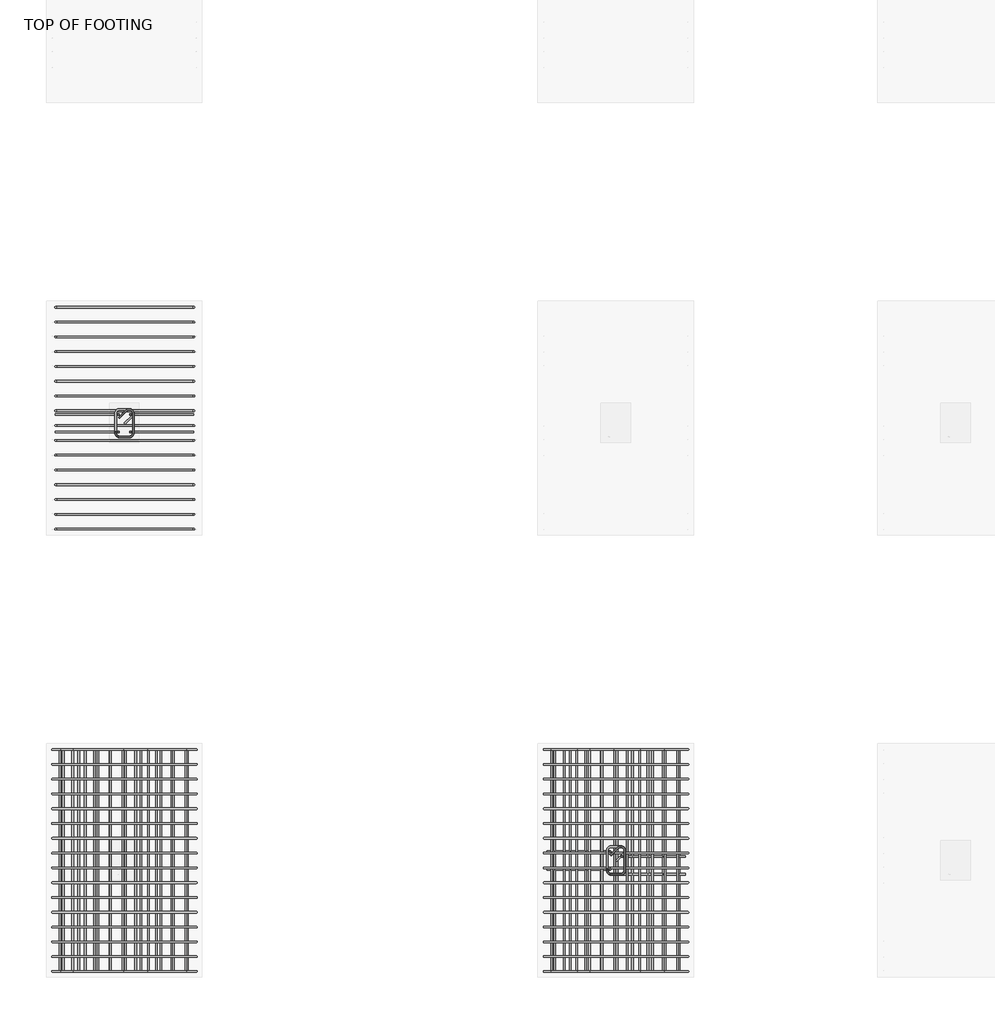
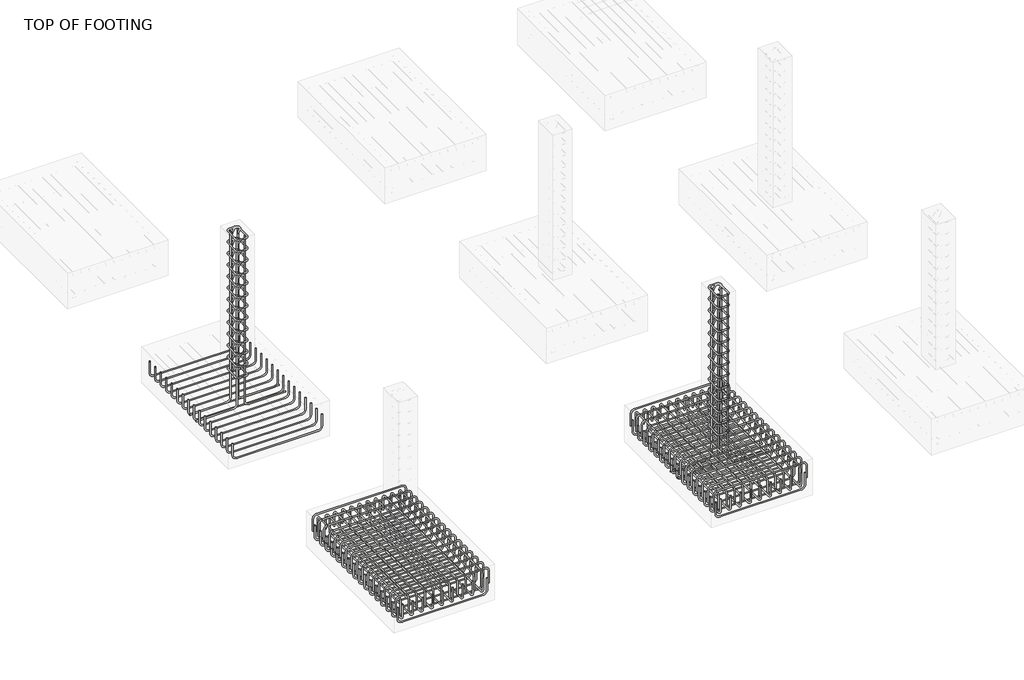
# One storey, part 5 of 8: 15 reinforcing bars.
"""IFC4 building model written with IfcOpenShell, lengths in millimetres."""

from ifc_helpers import new_model, si_unit, point, frame, origin, place, context, project, spatial, polyline, circle_curve, trimmed, segment, composite_curve, source, transform, mapped, element, save
from ifc_brep_helpers import swept_disk

model = new_model("IFC4")

# Units and contexts
model_context = context("Model", 3, world=origin())
ifc_project = project(units=[si_unit("LENGTHUNIT", "METRE", prefix="MILLI")], contexts=[model_context])

# Site, building, storey
site = spatial("IfcSite", under=ifc_project)
building = spatial("IfcBuilding", under=site)
storey = spatial("IfcBuildingStorey", under=building, Name="TOP OF FOOTING", Elevation=-1828.8)

# Reinforcing bars
placement = place(None, origin())
reinforcing_bar_shape = source(origin(), model_context, "Body", "SolidModel", [
    swept_disk(composite_curve([segment(polyline([(6846.0817577, 2235.4007933, -46.35), (6901.8253207, 2291.1443562, -46.35)]), True, "CONTINUOUS"), segment(trimmed(circle_curve(frame((6923.9931183, 2268.9765586, -46.35), z_axis=(0.0, 0.0, -1.0), x_axis=(-22.167797600000085, 22.167797600000085, 0.0)), 31.35), [point((6901.8253207, 2291.1443562, -46.35))], [point((6955.3431183, 2268.9765586, -46.35))], True, "CARTESIAN"), True, "CONTINUOUS"), segment(polyline([(6955.3431183, 2268.9765586, -46.35), (6955.3431183, 2119.5765586, -46.35)]), True, "CONTINUOUS"), segment(trimmed(circle_curve(frame((6923.9931183, 2119.5765586, -46.35), z_axis=(0.0, 0.0, -1.0), x_axis=(31.350000000000364, 0.0, 0.0)), 31.35), [point((6955.3431183, 2119.5765586, -46.35))], [point((6923.9931183, 2088.2265586, -46.35))], True, "CARTESIAN"), True, "CONTINUOUS"), segment(polyline([(6923.9931183, 2088.2265586, -46.35), (6850.7931183, 2088.2265586, -46.35)]), True, "CONTINUOUS"), segment(trimmed(circle_curve(frame((6850.7931183, 2119.5205096, -44.4761991), z_axis=(0.0, 0.05977036468717588, -0.9982121535551258), x_axis=(0.0, -31.293951000000106, -1.873800899999999)), 31.35), [point((6850.7931183, 2088.2265586, -46.35))], [point((6819.4431183, 2119.5205096, -44.4761991))], True, "CARTESIAN"), True, "CONTINUOUS"), segment(polyline([(6819.4431183, 2119.5205096, -44.4761991), (6819.4431183, 2269.0326076, -35.5238009)]), True, "CONTINUOUS"), segment(trimmed(circle_curve(frame((6850.7931183, 2269.0326076, -35.5238009), z_axis=(0.0, 0.05977036468717588, -0.9982121535551258), x_axis=(-31.350000000000364, 0.0, 0.0)), 31.35), [point((6819.4431183, 2269.0326076, -35.5238009))], [point((6850.7931183, 2300.3265586, -33.65))], True, "CARTESIAN"), True, "CONTINUOUS"), segment(polyline([(6850.7931183, 2300.3265586, -33.65), (6923.9931183, 2300.3265586, -33.65)]), True, "CONTINUOUS"), segment(trimmed(circle_curve(frame((6923.9931183, 2268.9765586, -33.65), z_axis=(0.0, 0.0, -1.0), x_axis=(0.0, 31.350000000000364, 0.0)), 31.35), [point((6923.9931183, 2300.3265586, -33.65))], [point((6946.1609159, 2246.808761, -33.65))], True, "CARTESIAN"), True, "CONTINUOUS"), segment(polyline([(6946.1609159, 2246.808761, -33.65), (6890.4173529, 2191.0651981, -33.65)]), True, "CONTINUOUS")], self_intersect=False), 6.35),
])
element("IfcReinforcingBar", 1, at=placement, inside=storey, context=model_context, shape_type="MappedRepresentation", body=[
    mapped(reinforcing_bar_shape, transform((0.0, 0.0, 0.0), x_axis=(1.0, 0.0, 0.0), y_axis=(0.0, 1.0, 0.0), z_axis=(0.0, 0.0, 1.0))),
    mapped(reinforcing_bar_shape, transform((0.0, 0.0, -144.675), x_axis=(1.0, 0.0, 0.0), y_axis=(0.0, 1.0, 0.0), z_axis=(0.0, 0.0, 1.0))),
    mapped(reinforcing_bar_shape, transform((0.0, 0.0, -289.35), x_axis=(1.0, 0.0, 0.0), y_axis=(0.0, 1.0, 0.0), z_axis=(0.0, 0.0, 1.0))),
    mapped(reinforcing_bar_shape, transform((0.0, 0.0, -434.025), x_axis=(1.0, 0.0, 0.0), y_axis=(0.0, 1.0, 0.0), z_axis=(0.0, 0.0, 1.0))),
    mapped(reinforcing_bar_shape, transform((0.0, 0.0, -578.7), x_axis=(1.0, 0.0, 0.0), y_axis=(0.0, 1.0, 0.0), z_axis=(0.0, 0.0, 1.0))),
    mapped(reinforcing_bar_shape, transform((0.0, 0.0, -723.375), x_axis=(1.0, 0.0, 0.0), y_axis=(0.0, 1.0, 0.0), z_axis=(0.0, 0.0, 1.0))),
    mapped(reinforcing_bar_shape, transform((0.0, 0.0, -868.05), x_axis=(1.0, 0.0, 0.0), y_axis=(0.0, 1.0, 0.0), z_axis=(0.0, 0.0, 1.0))),
    mapped(reinforcing_bar_shape, transform((0.0, 0.0, -1012.725), x_axis=(1.0, 0.0, 0.0), y_axis=(0.0, 1.0, 0.0), z_axis=(0.0, 0.0, 1.0))),
    mapped(reinforcing_bar_shape, transform((0.0, 0.0, -1157.4), x_axis=(1.0, 0.0, 0.0), y_axis=(0.0, 1.0, 0.0), z_axis=(0.0, 0.0, 1.0))),
    mapped(reinforcing_bar_shape, transform((0.0, 0.0, -1302.075), x_axis=(1.0, 0.0, 0.0), y_axis=(0.0, 1.0, 0.0), z_axis=(0.0, 0.0, 1.0))),
    mapped(reinforcing_bar_shape, transform((0.0, 0.0, -1446.75), x_axis=(1.0, 0.0, 0.0), y_axis=(0.0, 1.0, 0.0), z_axis=(0.0, 0.0, 1.0))),
    mapped(reinforcing_bar_shape, transform((0.0, 0.0, -1591.425), x_axis=(1.0, 0.0, 0.0), y_axis=(0.0, 1.0, 0.0), z_axis=(0.0, 0.0, 1.0))),
    mapped(reinforcing_bar_shape, transform((0.0, 0.0, -1736.1), x_axis=(1.0, 0.0, 0.0), y_axis=(0.0, 1.0, 0.0), z_axis=(0.0, 0.0, 1.0))),
])
reinforcing_bar_2_shape = source(origin(), model_context, "Body", "SolidModel", [
    swept_disk(composite_curve([segment(polyline([(7420.419602, 2088.2265586, -2177.1384798), (6979.2627797, 2088.2265586, -2177.1384798)]), True, "CONTINUOUS"), segment(trimmed(circle_curve(frame((6979.2627797, 2088.2265586, -2130.7884798), z_axis=(0.0, 1.0, 0.0), x_axis=(0.0, 0.0, -46.34999999999991)), 46.35), [point((6979.2627797, 2088.2265586, -2177.1384798))], [point((6932.9127797, 2088.2265586, -2130.7884798))], True, "CARTESIAN"), True, "CONTINUOUS"), segment(polyline([(6932.9127797, 2088.2265586, -2130.7884798), (6932.9127797, 2088.2265586, -40.0)]), True, "CONTINUOUS")], self_intersect=False), 6.35),
])
element("IfcReinforcingBar", 2, at=placement, inside=storey, context=model_context, shape_type="MappedRepresentation", body=[
    mapped(reinforcing_bar_2_shape, transform((0.0, 0.0, 0.0), x_axis=(1.0, 0.0, 0.0), y_axis=(0.0, 1.0, 0.0), z_axis=(0.0, 0.0, 1.0))),
    mapped(reinforcing_bar_2_shape, transform((0.0, 135.9, 0.0), x_axis=(1.0, 0.0, 0.0), y_axis=(0.0, 1.0, 0.0), z_axis=(0.0, 0.0, 1.0))),
])
reinforcing_bar_3_shape = source(origin(), model_context, "Body", "SolidModel", [
    swept_disk(composite_curve([segment(polyline([(6354.3666346, 2126.3265586, -2177.1384798), (6795.5234568, 2126.3265586, -2177.1384798)]), True, "CONTINUOUS"), segment(trimmed(circle_curve(frame((6795.5234568, 2126.3265586, -2130.7884798), z_axis=(0.0, -1.0, 0.0), x_axis=(0.0, 0.0, -46.34999999999991)), 46.35), [point((6795.5234568, 2126.3265586, -2177.1384798))], [point((6841.8734568, 2126.3265586, -2130.7884798))], True, "CARTESIAN"), True, "CONTINUOUS"), segment(polyline([(6841.8734568, 2126.3265586, -2130.7884798), (6841.8734568, 2126.3265586, -40.0)]), True, "CONTINUOUS")], self_intersect=False), 6.35),
])
element("IfcReinforcingBar", 3, at=placement, inside=storey, context=model_context, shape_type="MappedRepresentation", body=[
    mapped(reinforcing_bar_3_shape, transform((0.0, 0.0, 0.0), x_axis=(1.0, 0.0, 0.0), y_axis=(0.0, 1.0, 0.0), z_axis=(0.0, 0.0, 1.0))),
    mapped(reinforcing_bar_3_shape, transform((0.0, 135.9, 0.0), x_axis=(1.0, 0.0, 0.0), y_axis=(0.0, 1.0, 0.0), z_axis=(0.0, 0.0, 1.0))),
])
reinforcing_bar_4_shape = source(origin(), model_context, "Body", "SolidModel", [
    swept_disk(composite_curve([segment(polyline([(3061.4817577, 5600.7423139, -46.35), (3117.2253207, 5656.4858768, -46.35)]), True, "CONTINUOUS"), segment(trimmed(circle_curve(frame((3139.3931183, 5634.3180792, -46.35), z_axis=(0.0, 0.0, -1.0), x_axis=(-22.167797600000085, 22.167797600000085, 0.0)), 31.35), [point((3117.2253207, 5656.4858768, -46.35))], [point((3170.7431183, 5634.3180792, -46.35))], True, "CARTESIAN"), True, "CONTINUOUS"), segment(polyline([(3170.7431183, 5634.3180792, -46.35), (3170.7431183, 5484.9180792, -46.35)]), True, "CONTINUOUS"), segment(trimmed(circle_curve(frame((3139.3931183, 5484.9180792, -46.35), z_axis=(0.0, 0.0, -1.0), x_axis=(31.34999999999991, 0.0, 0.0)), 31.35), [point((3170.7431183, 5484.9180792, -46.35))], [point((3139.3931183, 5453.5680792, -46.35))], True, "CARTESIAN"), True, "CONTINUOUS"), segment(polyline([(3139.3931183, 5453.5680792, -46.35), (3066.1931183, 5453.5680792, -46.35)]), True, "CONTINUOUS"), segment(trimmed(circle_curve(frame((3066.1931183, 5484.8620303, -44.4761991), z_axis=(0.0, 0.05977036468717588, -0.9982121535551258), x_axis=(0.0, -31.293951099999504, -1.873800899999999)), 31.35), [point((3066.1931183, 5453.5680792, -46.35))], [point((3034.8431183, 5484.8620303, -44.4761991))], True, "CARTESIAN"), True, "CONTINUOUS"), segment(polyline([(3034.8431183, 5484.8620303, -44.4761991), (3034.8431183, 5634.3741282, -35.5238009)]), True, "CONTINUOUS"), segment(trimmed(circle_curve(frame((3066.1931183, 5634.3741282, -35.5238009), z_axis=(0.0, 0.05977036468717588, -0.9982121535551258), x_axis=(-31.350000000000364, 0.0, 0.0)), 31.35), [point((3034.8431183, 5634.3741282, -35.5238009))], [point((3066.1931183, 5665.6680792, -33.65))], True, "CARTESIAN"), True, "CONTINUOUS"), segment(polyline([(3066.1931183, 5665.6680792, -33.65), (3139.3931183, 5665.6680792, -33.65)]), True, "CONTINUOUS"), segment(trimmed(circle_curve(frame((3139.3931183, 5634.3180792, -33.65), z_axis=(0.0, 0.0, -1.0), x_axis=(0.0, 31.349999999999454, 0.0)), 31.35), [point((3139.3931183, 5665.6680792, -33.65))], [point((3161.5609159, 5612.1502816, -33.65))], True, "CARTESIAN"), True, "CONTINUOUS"), segment(polyline([(3161.5609159, 5612.1502816, -33.65), (3105.8173529, 5556.4067187, -33.65)]), True, "CONTINUOUS")], self_intersect=False), 6.35),
])
element("IfcReinforcingBar", 4, at=placement, inside=storey, context=model_context, shape_type="MappedRepresentation", body=[
    mapped(reinforcing_bar_4_shape, transform((0.0, 0.0, 0.0), x_axis=(1.0, 0.0, 0.0), y_axis=(0.0, 1.0, 0.0), z_axis=(0.0, 0.0, 1.0))),
    mapped(reinforcing_bar_4_shape, transform((0.0, 0.0, -144.675), x_axis=(1.0, 0.0, 0.0), y_axis=(0.0, 1.0, 0.0), z_axis=(0.0, 0.0, 1.0))),
    mapped(reinforcing_bar_4_shape, transform((0.0, 0.0, -289.35), x_axis=(1.0, 0.0, 0.0), y_axis=(0.0, 1.0, 0.0), z_axis=(0.0, 0.0, 1.0))),
    mapped(reinforcing_bar_4_shape, transform((0.0, 0.0, -434.025), x_axis=(1.0, 0.0, 0.0), y_axis=(0.0, 1.0, 0.0), z_axis=(0.0, 0.0, 1.0))),
    mapped(reinforcing_bar_4_shape, transform((0.0, 0.0, -578.7), x_axis=(1.0, 0.0, 0.0), y_axis=(0.0, 1.0, 0.0), z_axis=(0.0, 0.0, 1.0))),
    mapped(reinforcing_bar_4_shape, transform((0.0, 0.0, -723.375), x_axis=(1.0, 0.0, 0.0), y_axis=(0.0, 1.0, 0.0), z_axis=(0.0, 0.0, 1.0))),
    mapped(reinforcing_bar_4_shape, transform((0.0, 0.0, -868.05), x_axis=(1.0, 0.0, 0.0), y_axis=(0.0, 1.0, 0.0), z_axis=(0.0, 0.0, 1.0))),
    mapped(reinforcing_bar_4_shape, transform((0.0, 0.0, -1012.725), x_axis=(1.0, 0.0, 0.0), y_axis=(0.0, 1.0, 0.0), z_axis=(0.0, 0.0, 1.0))),
    mapped(reinforcing_bar_4_shape, transform((0.0, 0.0, -1157.4), x_axis=(1.0, 0.0, 0.0), y_axis=(0.0, 1.0, 0.0), z_axis=(0.0, 0.0, 1.0))),
    mapped(reinforcing_bar_4_shape, transform((0.0, 0.0, -1302.075), x_axis=(1.0, 0.0, 0.0), y_axis=(0.0, 1.0, 0.0), z_axis=(0.0, 0.0, 1.0))),
    mapped(reinforcing_bar_4_shape, transform((0.0, 0.0, -1446.75), x_axis=(1.0, 0.0, 0.0), y_axis=(0.0, 1.0, 0.0), z_axis=(0.0, 0.0, 1.0))),
    mapped(reinforcing_bar_4_shape, transform((0.0, 0.0, -1591.425), x_axis=(1.0, 0.0, 0.0), y_axis=(0.0, 1.0, 0.0), z_axis=(0.0, 0.0, 1.0))),
    mapped(reinforcing_bar_4_shape, transform((0.0, 0.0, -1736.1), x_axis=(1.0, 0.0, 0.0), y_axis=(0.0, 1.0, 0.0), z_axis=(0.0, 0.0, 1.0))),
])
reinforcing_bar_5_shape = source(origin(), model_context, "Body", "SolidModel", [
    swept_disk(composite_curve([segment(polyline([(3635.819602, 5491.6680792, -2177.1384798), (3194.6627797, 5491.6680792, -2177.1384798)]), True, "CONTINUOUS"), segment(trimmed(circle_curve(frame((3194.6627797, 5491.6680792, -2130.7884798), z_axis=(0.0, 1.0, 0.0), x_axis=(0.0, 0.0, -46.34999999999991)), 46.35), [point((3194.6627797, 5491.6680792, -2177.1384798))], [point((3148.3127797, 5491.6680792, -2130.7884798))], True, "CARTESIAN"), True, "CONTINUOUS"), segment(polyline([(3148.3127797, 5491.6680792, -2130.7884798), (3148.3127797, 5491.6680792, -40.0)]), True, "CONTINUOUS")], self_intersect=False), 6.35),
])
element("IfcReinforcingBar", 5, at=placement, inside=storey, context=model_context, shape_type="MappedRepresentation", body=[
    mapped(reinforcing_bar_5_shape, transform((0.0, 0.0, 0.0), x_axis=(1.0, 0.0, 0.0), y_axis=(0.0, 1.0, 0.0), z_axis=(0.0, 0.0, 1.0))),
    mapped(reinforcing_bar_5_shape, transform((0.0, 135.9, 0.0), x_axis=(1.0, 0.0, 0.0), y_axis=(0.0, 1.0, 0.0), z_axis=(0.0, 0.0, 1.0))),
])
reinforcing_bar_6_shape = source(origin(), model_context, "Body", "SolidModel", [
    swept_disk(composite_curve([segment(polyline([(2569.7666346, 5491.6680792, -2177.1384798), (3010.9234568, 5491.6680792, -2177.1384798)]), True, "CONTINUOUS"), segment(trimmed(circle_curve(frame((3010.9234568, 5491.6680792, -2130.7884798), z_axis=(0.0, -1.0, 0.0), x_axis=(0.0, 0.0, -46.34999999999991)), 46.35), [point((3010.9234568, 5491.6680792, -2177.1384798))], [point((3057.2734568, 5491.6680792, -2130.7884798))], True, "CARTESIAN"), True, "CONTINUOUS"), segment(polyline([(3057.2734568, 5491.6680792, -2130.7884798), (3057.2734568, 5491.6680792, -40.0)]), True, "CONTINUOUS")], self_intersect=False), 6.35),
])
element("IfcReinforcingBar", 6, at=placement, inside=storey, context=model_context, shape_type="MappedRepresentation", body=[
    mapped(reinforcing_bar_6_shape, transform((0.0, 0.0, 0.0), x_axis=(1.0, 0.0, 0.0), y_axis=(0.0, 1.0, 0.0), z_axis=(0.0, 0.0, 1.0))),
    mapped(reinforcing_bar_6_shape, transform((0.0, 135.9, 0.0), x_axis=(1.0, 0.0, 0.0), y_axis=(0.0, 1.0, 0.0), z_axis=(0.0, 0.0, 1.0))),
])
reinforcing_bar_7_shape = source(origin(), model_context, "Body", "SolidModel", [
    swept_disk(composite_curve([segment(polyline([(3637.0426771, 3047.9265586, -2008.2544267), (3637.0426771, 3047.9265586, -2155.5544267)]), True, "CONTINUOUS"), segment(trimmed(circle_curve(frame((3590.6926771, 3047.9265586, -2155.5544267), z_axis=(0.0, 1.0, 0.0), x_axis=(46.350000000000364, 0.0, 0.0)), 46.35), [point((3637.0426771, 3047.9265586, -2155.5544267))], [point((3590.6926771, 3047.9265586, -2201.9044267))], True, "CARTESIAN"), True, "CONTINUOUS"), segment(polyline([(3590.6926771, 3047.9265586, -2201.9044267), (2619.6766408, 3047.9265586, -2201.9044267)]), True, "CONTINUOUS"), segment(trimmed(circle_curve(frame((2619.6766408, 3047.9265586, -2155.5544267), z_axis=(0.0, 1.0, 0.0), x_axis=(0.0, 0.0, -46.34999999999991)), 46.35), [point((2619.6766408, 3047.9265586, -2201.9044267))], [point((2573.3266408, 3047.9265586, -2155.5544267))], True, "CARTESIAN"), True, "CONTINUOUS"), segment(polyline([(2573.3266408, 3047.9265586, -2155.5544267), (2573.3266408, 3047.9265586, -2008.2544267)]), True, "CONTINUOUS")], self_intersect=False), 6.35),
])
element("IfcReinforcingBar", 7, at=placement, inside=storey, context=model_context, shape_type="MappedRepresentation", body=[
    mapped(reinforcing_bar_7_shape, transform((0.0, 0.0, 0.0), x_axis=(1.0, 0.0, 0.0), y_axis=(0.0, 1.0, 0.0), z_axis=(0.0, 0.0, 1.0))),
    mapped(reinforcing_bar_7_shape, transform((0.0, -113.82, 0.0), x_axis=(1.0, 0.0, 0.0), y_axis=(0.0, 1.0, 0.0), z_axis=(0.0, 0.0, 1.0))),
    mapped(reinforcing_bar_7_shape, transform((0.0, -227.64, 0.0), x_axis=(1.0, 0.0, 0.0), y_axis=(0.0, 1.0, 0.0), z_axis=(0.0, 0.0, 1.0))),
    mapped(reinforcing_bar_7_shape, transform((0.0, -341.46, 0.0), x_axis=(1.0, 0.0, 0.0), y_axis=(0.0, 1.0, 0.0), z_axis=(0.0, 0.0, 1.0))),
    mapped(reinforcing_bar_7_shape, transform((0.0, -455.28, 0.0), x_axis=(1.0, 0.0, 0.0), y_axis=(0.0, 1.0, 0.0), z_axis=(0.0, 0.0, 1.0))),
    mapped(reinforcing_bar_7_shape, transform((0.0, -569.1, 0.0), x_axis=(1.0, 0.0, 0.0), y_axis=(0.0, 1.0, 0.0), z_axis=(0.0, 0.0, 1.0))),
    mapped(reinforcing_bar_7_shape, transform((0.0, -682.92, 0.0), x_axis=(1.0, 0.0, 0.0), y_axis=(0.0, 1.0, 0.0), z_axis=(0.0, 0.0, 1.0))),
    mapped(reinforcing_bar_7_shape, transform((0.0, -796.74, 0.0), x_axis=(1.0, 0.0, 0.0), y_axis=(0.0, 1.0, 0.0), z_axis=(0.0, 0.0, 1.0))),
    mapped(reinforcing_bar_7_shape, transform((0.0, -910.56, 0.0), x_axis=(1.0, 0.0, 0.0), y_axis=(0.0, 1.0, 0.0), z_axis=(0.0, 0.0, 1.0))),
    mapped(reinforcing_bar_7_shape, transform((0.0, -1024.38, 0.0), x_axis=(1.0, 0.0, 0.0), y_axis=(0.0, 1.0, 0.0), z_axis=(0.0, 0.0, 1.0))),
    mapped(reinforcing_bar_7_shape, transform((0.0, -1138.2, 0.0), x_axis=(1.0, 0.0, 0.0), y_axis=(0.0, 1.0, 0.0), z_axis=(0.0, 0.0, 1.0))),
    mapped(reinforcing_bar_7_shape, transform((0.0, -1252.02, 0.0), x_axis=(1.0, 0.0, 0.0), y_axis=(0.0, 1.0, 0.0), z_axis=(0.0, 0.0, 1.0))),
    mapped(reinforcing_bar_7_shape, transform((0.0, -1365.84, 0.0), x_axis=(1.0, 0.0, 0.0), y_axis=(0.0, 1.0, 0.0), z_axis=(0.0, 0.0, 1.0))),
    mapped(reinforcing_bar_7_shape, transform((0.0, -1479.66, 0.0), x_axis=(1.0, 0.0, 0.0), y_axis=(0.0, 1.0, 0.0), z_axis=(0.0, 0.0, 1.0))),
    mapped(reinforcing_bar_7_shape, transform((0.0, -1593.48, 0.0), x_axis=(1.0, 0.0, 0.0), y_axis=(0.0, 1.0, 0.0), z_axis=(0.0, 0.0, 1.0))),
    mapped(reinforcing_bar_7_shape, transform((0.0, -1707.3, 0.0), x_axis=(1.0, 0.0, 0.0), y_axis=(0.0, 1.0, 0.0), z_axis=(0.0, 0.0, 1.0))),
])
reinforcing_bar_8_shape = source(origin(), model_context, "Body", "SolidModel", [
    swept_disk(composite_curve([segment(polyline([(2549.1431183, 3047.9265586, -2068.8), (2549.1431183, 3047.9265586, -1921.5)]), True, "CONTINUOUS"), segment(trimmed(circle_curve(frame((2595.4931183, 3047.9265586, -1921.5), z_axis=(0.0, 1.0, 0.0), x_axis=(-46.34999999999991, 0.0, 0.0)), 46.35), [point((2549.1431183, 3047.9265586, -1921.5))], [point((2595.4931183, 3047.9265586, -1875.15))], True, "CARTESIAN"), True, "CONTINUOUS"), segment(polyline([(2595.4931183, 3047.9265586, -1875.15), (3610.0931183, 3047.9265586, -1875.15)]), True, "CONTINUOUS"), segment(trimmed(circle_curve(frame((3610.0931183, 3047.9265586, -1921.5), z_axis=(0.0, 1.0, 0.0), x_axis=(0.0, 0.0, 46.34999999999991)), 46.35), [point((3610.0931183, 3047.9265586, -1875.15))], [point((3656.4431183, 3047.9265586, -1921.5))], True, "CARTESIAN"), True, "CONTINUOUS"), segment(polyline([(3656.4431183, 3047.9265586, -1921.5), (3656.4431183, 3047.9265586, -2068.8)]), True, "CONTINUOUS")], self_intersect=False), 6.35),
])
element("IfcReinforcingBar", 8, at=placement, inside=storey, context=model_context, shape_type="MappedRepresentation", body=[
    mapped(reinforcing_bar_8_shape, transform((0.0, 0.0, 0.0), x_axis=(1.0, 0.0, 0.0), y_axis=(0.0, 1.0, 0.0), z_axis=(0.0, 0.0, 1.0))),
    mapped(reinforcing_bar_8_shape, transform((0.0, -113.82, 0.0), x_axis=(1.0, 0.0, 0.0), y_axis=(0.0, 1.0, 0.0), z_axis=(0.0, 0.0, 1.0))),
    mapped(reinforcing_bar_8_shape, transform((0.0, -227.64, 0.0), x_axis=(1.0, 0.0, 0.0), y_axis=(0.0, 1.0, 0.0), z_axis=(0.0, 0.0, 1.0))),
    mapped(reinforcing_bar_8_shape, transform((0.0, -341.46, 0.0), x_axis=(1.0, 0.0, 0.0), y_axis=(0.0, 1.0, 0.0), z_axis=(0.0, 0.0, 1.0))),
    mapped(reinforcing_bar_8_shape, transform((0.0, -455.28, 0.0), x_axis=(1.0, 0.0, 0.0), y_axis=(0.0, 1.0, 0.0), z_axis=(0.0, 0.0, 1.0))),
    mapped(reinforcing_bar_8_shape, transform((0.0, -569.1, 0.0), x_axis=(1.0, 0.0, 0.0), y_axis=(0.0, 1.0, 0.0), z_axis=(0.0, 0.0, 1.0))),
    mapped(reinforcing_bar_8_shape, transform((0.0, -682.92, 0.0), x_axis=(1.0, 0.0, 0.0), y_axis=(0.0, 1.0, 0.0), z_axis=(0.0, 0.0, 1.0))),
    mapped(reinforcing_bar_8_shape, transform((0.0, -796.74, 0.0), x_axis=(1.0, 0.0, 0.0), y_axis=(0.0, 1.0, 0.0), z_axis=(0.0, 0.0, 1.0))),
    mapped(reinforcing_bar_8_shape, transform((0.0, -910.56, 0.0), x_axis=(1.0, 0.0, 0.0), y_axis=(0.0, 1.0, 0.0), z_axis=(0.0, 0.0, 1.0))),
    mapped(reinforcing_bar_8_shape, transform((0.0, -1024.38, 0.0), x_axis=(1.0, 0.0, 0.0), y_axis=(0.0, 1.0, 0.0), z_axis=(0.0, 0.0, 1.0))),
    mapped(reinforcing_bar_8_shape, transform((0.0, -1138.2, 0.0), x_axis=(1.0, 0.0, 0.0), y_axis=(0.0, 1.0, 0.0), z_axis=(0.0, 0.0, 1.0))),
    mapped(reinforcing_bar_8_shape, transform((0.0, -1252.02, 0.0), x_axis=(1.0, 0.0, 0.0), y_axis=(0.0, 1.0, 0.0), z_axis=(0.0, 0.0, 1.0))),
    mapped(reinforcing_bar_8_shape, transform((0.0, -1365.84, 0.0), x_axis=(1.0, 0.0, 0.0), y_axis=(0.0, 1.0, 0.0), z_axis=(0.0, 0.0, 1.0))),
    mapped(reinforcing_bar_8_shape, transform((0.0, -1479.66, 0.0), x_axis=(1.0, 0.0, 0.0), y_axis=(0.0, 1.0, 0.0), z_axis=(0.0, 0.0, 1.0))),
    mapped(reinforcing_bar_8_shape, transform((0.0, -1593.48, 0.0), x_axis=(1.0, 0.0, 0.0), y_axis=(0.0, 1.0, 0.0), z_axis=(0.0, 0.0, 1.0))),
    mapped(reinforcing_bar_8_shape, transform((0.0, -1707.3, 0.0), x_axis=(1.0, 0.0, 0.0), y_axis=(0.0, 1.0, 0.0), z_axis=(0.0, 0.0, 1.0))),
])
reinforcing_bar_9_shape = source(origin(), model_context, "Body", "SolidModel", [
    swept_disk(composite_curve([segment(polyline([(2631.3651697, 3047.9265586, -1986.9111268), (2631.3651697, 3047.9265586, -2134.2111268)]), True, "CONTINUOUS"), segment(trimmed(circle_curve(frame((2631.3651697, 3001.5765586, -2134.2111268), z_axis=(-1.0, 0.0, 0.0), x_axis=(0.0, 46.34999999999991, 0.0)), 46.35), [point((2631.3651697, 3047.9265586, -2134.2111268))], [point((2631.3651697, 3001.5765586, -2180.5611268))], True, "CARTESIAN"), True, "CONTINUOUS"), segment(polyline([(2631.3651697, 3001.5765586, -2180.5611268), (2631.3651697, 1386.9765586, -2180.5611268)]), True, "CONTINUOUS"), segment(trimmed(circle_curve(frame((2631.3651697, 1386.9765586, -2134.2111268), z_axis=(-1.0, 0.0, 0.0), x_axis=(0.0, 0.0, -46.34999999999991)), 46.35), [point((2631.3651697, 1386.9765586, -2180.5611268))], [point((2631.3651697, 1340.6265586, -2134.2111268))], True, "CARTESIAN"), True, "CONTINUOUS"), segment(polyline([(2631.3651697, 1340.6265586, -2134.2111268), (2631.3651697, 1340.6265586, -1986.9111268)]), True, "CONTINUOUS")], self_intersect=False), 6.35),
])
element("IfcReinforcingBar", 9, at=placement, inside=storey, context=model_context, shape_type="MappedRepresentation", body=[
    mapped(reinforcing_bar_9_shape, transform((0.0, 0.0, 0.0), x_axis=(1.0, 0.0, 0.0), y_axis=(0.0, 1.0, 0.0), z_axis=(0.0, 0.0, 1.0))),
    mapped(reinforcing_bar_9_shape, transform((119.5564677, 0.0, 0.0), x_axis=(1.0, 0.0, 0.0), y_axis=(0.0, 1.0, 0.0), z_axis=(0.0, 0.0, 1.0))),
    mapped(reinforcing_bar_9_shape, transform((239.1129355, 0.0, 0.0), x_axis=(1.0, 0.0, 0.0), y_axis=(0.0, 1.0, 0.0), z_axis=(0.0, 0.0, 1.0))),
    mapped(reinforcing_bar_9_shape, transform((358.6694032, 0.0, 0.0), x_axis=(1.0, 0.0, 0.0), y_axis=(0.0, 1.0, 0.0), z_axis=(0.0, 0.0, 1.0))),
    mapped(reinforcing_bar_9_shape, transform((478.2258709, 0.0, 0.0), x_axis=(1.0, 0.0, 0.0), y_axis=(0.0, 1.0, 0.0), z_axis=(0.0, 0.0, 1.0))),
    mapped(reinforcing_bar_9_shape, transform((597.7823387, 0.0, 0.0), x_axis=(1.0, 0.0, 0.0), y_axis=(0.0, 1.0, 0.0), z_axis=(0.0, 0.0, 1.0))),
    mapped(reinforcing_bar_9_shape, transform((717.3388064, 0.0, 0.0), x_axis=(1.0, 0.0, 0.0), y_axis=(0.0, 1.0, 0.0), z_axis=(0.0, 0.0, 1.0))),
    mapped(reinforcing_bar_9_shape, transform((836.8952741, 0.0, 0.0), x_axis=(1.0, 0.0, 0.0), y_axis=(0.0, 1.0, 0.0), z_axis=(0.0, 0.0, 1.0))),
    mapped(reinforcing_bar_9_shape, transform((956.4517419, 0.0, 0.0), x_axis=(1.0, 0.0, 0.0), y_axis=(0.0, 1.0, 0.0), z_axis=(0.0, 0.0, 1.0))),
])
reinforcing_bar_10_shape = source(origin(), model_context, "Body", "SolidModel", [
    swept_disk(composite_curve([segment(polyline([(3577.1331701, 3047.9265586, -2094.8977257), (3577.1331701, 3047.9265586, -1947.5977257)]), True, "CONTINUOUS"), segment(trimmed(circle_curve(frame((3577.1331701, 3001.5765586, -1947.5977257), z_axis=(1.0, 0.0, 0.0), x_axis=(0.0, 46.34999999999991, 0.0)), 46.35), [point((3577.1331701, 3047.9265586, -1947.5977257))], [point((3577.1331701, 3001.5765586, -1901.2477257))], True, "CARTESIAN"), True, "CONTINUOUS"), segment(polyline([(3577.1331701, 3001.5765586, -1901.2477257), (3577.1331701, 1386.9765586, -1901.2477257)]), True, "CONTINUOUS"), segment(trimmed(circle_curve(frame((3577.1331701, 1386.9765586, -1947.5977257), z_axis=(1.0, 0.0, 0.0), x_axis=(0.0, 0.0, 46.34999999999991)), 46.35), [point((3577.1331701, 1386.9765586, -1901.2477257))], [point((3577.1331701, 1340.6265586, -1947.5977257))], True, "CARTESIAN"), True, "CONTINUOUS"), segment(polyline([(3577.1331701, 1340.6265586, -1947.5977257), (3577.1331701, 1340.6265586, -2094.8977257)]), True, "CONTINUOUS")], self_intersect=False), 6.35),
])
element("IfcReinforcingBar", 10, at=placement, inside=storey, context=model_context, shape_type="MappedRepresentation", body=[
    mapped(reinforcing_bar_10_shape, transform((0.0, 0.0, 0.0), x_axis=(1.0, 0.0, 0.0), y_axis=(0.0, 1.0, 0.0), z_axis=(0.0, 0.0, 1.0))),
    mapped(reinforcing_bar_10_shape, transform((-97.0050815, 0.0, 0.0), x_axis=(1.0, 0.0, 0.0), y_axis=(0.0, 1.0, 0.0), z_axis=(0.0, 0.0, 1.0))),
    mapped(reinforcing_bar_10_shape, transform((-194.0101631, 0.0, 0.0), x_axis=(1.0, 0.0, 0.0), y_axis=(0.0, 1.0, 0.0), z_axis=(0.0, 0.0, 1.0))),
    mapped(reinforcing_bar_10_shape, transform((-291.0152446, 0.0, 0.0), x_axis=(1.0, 0.0, 0.0), y_axis=(0.0, 1.0, 0.0), z_axis=(0.0, 0.0, 1.0))),
    mapped(reinforcing_bar_10_shape, transform((-388.0203261, 0.0, 0.0), x_axis=(1.0, 0.0, 0.0), y_axis=(0.0, 1.0, 0.0), z_axis=(0.0, 0.0, 1.0))),
    mapped(reinforcing_bar_10_shape, transform((-485.0254076, 0.0, 0.0), x_axis=(1.0, 0.0, 0.0), y_axis=(0.0, 1.0, 0.0), z_axis=(0.0, 0.0, 1.0))),
    mapped(reinforcing_bar_10_shape, transform((-582.0304892, 0.0, 0.0), x_axis=(1.0, 0.0, 0.0), y_axis=(0.0, 1.0, 0.0), z_axis=(0.0, 0.0, 1.0))),
    mapped(reinforcing_bar_10_shape, transform((-679.0355707, 0.0, 0.0), x_axis=(1.0, 0.0, 0.0), y_axis=(0.0, 1.0, 0.0), z_axis=(0.0, 0.0, 1.0))),
    mapped(reinforcing_bar_10_shape, transform((-776.0406522, 0.0, 0.0), x_axis=(1.0, 0.0, 0.0), y_axis=(0.0, 1.0, 0.0), z_axis=(0.0, 0.0, 1.0))),
    mapped(reinforcing_bar_10_shape, transform((-873.0457338, 0.0, 0.0), x_axis=(1.0, 0.0, 0.0), y_axis=(0.0, 1.0, 0.0), z_axis=(0.0, 0.0, 1.0))),
    mapped(reinforcing_bar_10_shape, transform((-970.0508153, 0.0, 0.0), x_axis=(1.0, 0.0, 0.0), y_axis=(0.0, 1.0, 0.0), z_axis=(0.0, 0.0, 1.0))),
])
reinforcing_bar_11_shape = source(origin(), model_context, "Body", "SolidModel", [
    swept_disk(composite_curve([segment(polyline([(3637.0426771, 6451.7662126, -2008.2544267), (3637.0426771, 6451.7662126, -2155.5544267)]), True, "CONTINUOUS"), segment(trimmed(circle_curve(frame((3590.6926771, 6451.7662126, -2155.5544267), z_axis=(0.0, 1.0, 0.0), x_axis=(46.350000000000364, 0.0, 0.0)), 46.35), [point((3637.0426771, 6451.7662126, -2155.5544267))], [point((3590.6926771, 6451.7662126, -2201.9044267))], True, "CARTESIAN"), True, "CONTINUOUS"), segment(polyline([(3590.6926771, 6451.7662126, -2201.9044267), (2619.6766408, 6451.7662126, -2201.9044267)]), True, "CONTINUOUS"), segment(trimmed(circle_curve(frame((2619.6766408, 6451.7662126, -2155.5544267), z_axis=(0.0, 1.0, 0.0), x_axis=(0.0, 0.0, -46.34999999999991)), 46.35), [point((2619.6766408, 6451.7662126, -2201.9044267))], [point((2573.3266408, 6451.7662126, -2155.5544267))], True, "CARTESIAN"), True, "CONTINUOUS"), segment(polyline([(2573.3266408, 6451.7662126, -2155.5544267), (2573.3266408, 6451.7662126, -2008.2544267)]), True, "CONTINUOUS")], self_intersect=False), 6.35),
])
element("IfcReinforcingBar", 11, at=placement, inside=storey, context=model_context, shape_type="MappedRepresentation", body=[
    mapped(reinforcing_bar_11_shape, transform((0.0, 0.0, 0.0), x_axis=(1.0, 0.0, 0.0), y_axis=(0.0, 1.0, 0.0), z_axis=(0.0, 0.0, 1.0))),
    mapped(reinforcing_bar_11_shape, transform((0.0, -113.82, 0.0), x_axis=(1.0, 0.0, 0.0), y_axis=(0.0, 1.0, 0.0), z_axis=(0.0, 0.0, 1.0))),
    mapped(reinforcing_bar_11_shape, transform((0.0, -227.64, 0.0), x_axis=(1.0, 0.0, 0.0), y_axis=(0.0, 1.0, 0.0), z_axis=(0.0, 0.0, 1.0))),
    mapped(reinforcing_bar_11_shape, transform((0.0, -341.46, 0.0), x_axis=(1.0, 0.0, 0.0), y_axis=(0.0, 1.0, 0.0), z_axis=(0.0, 0.0, 1.0))),
    mapped(reinforcing_bar_11_shape, transform((0.0, -455.28, 0.0), x_axis=(1.0, 0.0, 0.0), y_axis=(0.0, 1.0, 0.0), z_axis=(0.0, 0.0, 1.0))),
    mapped(reinforcing_bar_11_shape, transform((0.0, -569.1, 0.0), x_axis=(1.0, 0.0, 0.0), y_axis=(0.0, 1.0, 0.0), z_axis=(0.0, 0.0, 1.0))),
    mapped(reinforcing_bar_11_shape, transform((0.0, -682.92, 0.0), x_axis=(1.0, 0.0, 0.0), y_axis=(0.0, 1.0, 0.0), z_axis=(0.0, 0.0, 1.0))),
    mapped(reinforcing_bar_11_shape, transform((0.0, -796.74, 0.0), x_axis=(1.0, 0.0, 0.0), y_axis=(0.0, 1.0, 0.0), z_axis=(0.0, 0.0, 1.0))),
    mapped(reinforcing_bar_11_shape, transform((0.0, -910.56, 0.0), x_axis=(1.0, 0.0, 0.0), y_axis=(0.0, 1.0, 0.0), z_axis=(0.0, 0.0, 1.0))),
    mapped(reinforcing_bar_11_shape, transform((0.0, -1024.38, 0.0), x_axis=(1.0, 0.0, 0.0), y_axis=(0.0, 1.0, 0.0), z_axis=(0.0, 0.0, 1.0))),
    mapped(reinforcing_bar_11_shape, transform((0.0, -1138.2, 0.0), x_axis=(1.0, 0.0, 0.0), y_axis=(0.0, 1.0, 0.0), z_axis=(0.0, 0.0, 1.0))),
    mapped(reinforcing_bar_11_shape, transform((0.0, -1252.02, 0.0), x_axis=(1.0, 0.0, 0.0), y_axis=(0.0, 1.0, 0.0), z_axis=(0.0, 0.0, 1.0))),
    mapped(reinforcing_bar_11_shape, transform((0.0, -1365.84, 0.0), x_axis=(1.0, 0.0, 0.0), y_axis=(0.0, 1.0, 0.0), z_axis=(0.0, 0.0, 1.0))),
    mapped(reinforcing_bar_11_shape, transform((0.0, -1479.66, 0.0), x_axis=(1.0, 0.0, 0.0), y_axis=(0.0, 1.0, 0.0), z_axis=(0.0, 0.0, 1.0))),
    mapped(reinforcing_bar_11_shape, transform((0.0, -1593.48, 0.0), x_axis=(1.0, 0.0, 0.0), y_axis=(0.0, 1.0, 0.0), z_axis=(0.0, 0.0, 1.0))),
    mapped(reinforcing_bar_11_shape, transform((0.0, -1707.3, 0.0), x_axis=(1.0, 0.0, 0.0), y_axis=(0.0, 1.0, 0.0), z_axis=(0.0, 0.0, 1.0))),
])
reinforcing_bar_12_shape = source(origin(), model_context, "Body", "SolidModel", [
    swept_disk(composite_curve([segment(polyline([(7421.6426771, 3047.9265586, -2008.2544267), (7421.6426771, 3047.9265586, -2155.5544267)]), True, "CONTINUOUS"), segment(trimmed(circle_curve(frame((7375.2926771, 3047.9265586, -2155.5544267), z_axis=(0.0, 1.0, 0.0), x_axis=(46.349999999999454, 0.0, 0.0)), 46.35), [point((7421.6426771, 3047.9265586, -2155.5544267))], [point((7375.2926771, 3047.9265586, -2201.9044267))], True, "CARTESIAN"), True, "CONTINUOUS"), segment(polyline([(7375.2926771, 3047.9265586, -2201.9044267), (6404.2766408, 3047.9265586, -2201.9044267)]), True, "CONTINUOUS"), segment(trimmed(circle_curve(frame((6404.2766408, 3047.9265586, -2155.5544267), z_axis=(0.0, 1.0, 0.0), x_axis=(0.0, 0.0, -46.34999999999991)), 46.35), [point((6404.2766408, 3047.9265586, -2201.9044267))], [point((6357.9266408, 3047.9265586, -2155.5544267))], True, "CARTESIAN"), True, "CONTINUOUS"), segment(polyline([(6357.9266408, 3047.9265586, -2155.5544267), (6357.9266408, 3047.9265586, -2008.2544267)]), True, "CONTINUOUS")], self_intersect=False), 6.35),
])
element("IfcReinforcingBar", 12, at=placement, inside=storey, context=model_context, shape_type="MappedRepresentation", body=[
    mapped(reinforcing_bar_12_shape, transform((0.0, 0.0, 0.0), x_axis=(1.0, 0.0, 0.0), y_axis=(0.0, 1.0, 0.0), z_axis=(0.0, 0.0, 1.0))),
    mapped(reinforcing_bar_12_shape, transform((0.0, -113.82, 0.0), x_axis=(1.0, 0.0, 0.0), y_axis=(0.0, 1.0, 0.0), z_axis=(0.0, 0.0, 1.0))),
    mapped(reinforcing_bar_12_shape, transform((0.0, -227.64, 0.0), x_axis=(1.0, 0.0, 0.0), y_axis=(0.0, 1.0, 0.0), z_axis=(0.0, 0.0, 1.0))),
    mapped(reinforcing_bar_12_shape, transform((0.0, -341.46, 0.0), x_axis=(1.0, 0.0, 0.0), y_axis=(0.0, 1.0, 0.0), z_axis=(0.0, 0.0, 1.0))),
    mapped(reinforcing_bar_12_shape, transform((0.0, -455.28, 0.0), x_axis=(1.0, 0.0, 0.0), y_axis=(0.0, 1.0, 0.0), z_axis=(0.0, 0.0, 1.0))),
    mapped(reinforcing_bar_12_shape, transform((0.0, -569.1, 0.0), x_axis=(1.0, 0.0, 0.0), y_axis=(0.0, 1.0, 0.0), z_axis=(0.0, 0.0, 1.0))),
    mapped(reinforcing_bar_12_shape, transform((0.0, -682.92, 0.0), x_axis=(1.0, 0.0, 0.0), y_axis=(0.0, 1.0, 0.0), z_axis=(0.0, 0.0, 1.0))),
    mapped(reinforcing_bar_12_shape, transform((0.0, -796.74, 0.0), x_axis=(1.0, 0.0, 0.0), y_axis=(0.0, 1.0, 0.0), z_axis=(0.0, 0.0, 1.0))),
    mapped(reinforcing_bar_12_shape, transform((0.0, -910.56, 0.0), x_axis=(1.0, 0.0, 0.0), y_axis=(0.0, 1.0, 0.0), z_axis=(0.0, 0.0, 1.0))),
    mapped(reinforcing_bar_12_shape, transform((0.0, -1024.38, 0.0), x_axis=(1.0, 0.0, 0.0), y_axis=(0.0, 1.0, 0.0), z_axis=(0.0, 0.0, 1.0))),
    mapped(reinforcing_bar_12_shape, transform((0.0, -1138.2, 0.0), x_axis=(1.0, 0.0, 0.0), y_axis=(0.0, 1.0, 0.0), z_axis=(0.0, 0.0, 1.0))),
    mapped(reinforcing_bar_12_shape, transform((0.0, -1252.02, 0.0), x_axis=(1.0, 0.0, 0.0), y_axis=(0.0, 1.0, 0.0), z_axis=(0.0, 0.0, 1.0))),
    mapped(reinforcing_bar_12_shape, transform((0.0, -1365.84, 0.0), x_axis=(1.0, 0.0, 0.0), y_axis=(0.0, 1.0, 0.0), z_axis=(0.0, 0.0, 1.0))),
    mapped(reinforcing_bar_12_shape, transform((0.0, -1479.66, 0.0), x_axis=(1.0, 0.0, 0.0), y_axis=(0.0, 1.0, 0.0), z_axis=(0.0, 0.0, 1.0))),
    mapped(reinforcing_bar_12_shape, transform((0.0, -1593.48, 0.0), x_axis=(1.0, 0.0, 0.0), y_axis=(0.0, 1.0, 0.0), z_axis=(0.0, 0.0, 1.0))),
    mapped(reinforcing_bar_12_shape, transform((0.0, -1707.3, 0.0), x_axis=(1.0, 0.0, 0.0), y_axis=(0.0, 1.0, 0.0), z_axis=(0.0, 0.0, 1.0))),
])
reinforcing_bar_13_shape = source(origin(), model_context, "Body", "SolidModel", [
    swept_disk(composite_curve([segment(polyline([(6333.7431183, 3047.9265586, -2068.8), (6333.7431183, 3047.9265586, -1921.5)]), True, "CONTINUOUS"), segment(trimmed(circle_curve(frame((6380.0931183, 3047.9265586, -1921.5), z_axis=(0.0, 1.0, 0.0), x_axis=(-46.350000000000364, 0.0, 0.0)), 46.35), [point((6333.7431183, 3047.9265586, -1921.5))], [point((6380.0931183, 3047.9265586, -1875.15))], True, "CARTESIAN"), True, "CONTINUOUS"), segment(polyline([(6380.0931183, 3047.9265586, -1875.15), (7394.6931183, 3047.9265586, -1875.15)]), True, "CONTINUOUS"), segment(trimmed(circle_curve(frame((7394.6931183, 3047.9265586, -1921.5), z_axis=(0.0, 1.0, 0.0), x_axis=(0.0, 0.0, 46.34999999999991)), 46.35), [point((7394.6931183, 3047.9265586, -1875.15))], [point((7441.0431183, 3047.9265586, -1921.5))], True, "CARTESIAN"), True, "CONTINUOUS"), segment(polyline([(7441.0431183, 3047.9265586, -1921.5), (7441.0431183, 3047.9265586, -2068.8)]), True, "CONTINUOUS")], self_intersect=False), 6.35),
])
element("IfcReinforcingBar", 13, at=placement, inside=storey, context=model_context, shape_type="MappedRepresentation", body=[
    mapped(reinforcing_bar_13_shape, transform((0.0, 0.0, 0.0), x_axis=(1.0, 0.0, 0.0), y_axis=(0.0, 1.0, 0.0), z_axis=(0.0, 0.0, 1.0))),
    mapped(reinforcing_bar_13_shape, transform((0.0, -113.82, 0.0), x_axis=(1.0, 0.0, 0.0), y_axis=(0.0, 1.0, 0.0), z_axis=(0.0, 0.0, 1.0))),
    mapped(reinforcing_bar_13_shape, transform((0.0, -227.64, 0.0), x_axis=(1.0, 0.0, 0.0), y_axis=(0.0, 1.0, 0.0), z_axis=(0.0, 0.0, 1.0))),
    mapped(reinforcing_bar_13_shape, transform((0.0, -341.46, 0.0), x_axis=(1.0, 0.0, 0.0), y_axis=(0.0, 1.0, 0.0), z_axis=(0.0, 0.0, 1.0))),
    mapped(reinforcing_bar_13_shape, transform((0.0, -455.28, 0.0), x_axis=(1.0, 0.0, 0.0), y_axis=(0.0, 1.0, 0.0), z_axis=(0.0, 0.0, 1.0))),
    mapped(reinforcing_bar_13_shape, transform((0.0, -569.1, 0.0), x_axis=(1.0, 0.0, 0.0), y_axis=(0.0, 1.0, 0.0), z_axis=(0.0, 0.0, 1.0))),
    mapped(reinforcing_bar_13_shape, transform((0.0, -682.92, 0.0), x_axis=(1.0, 0.0, 0.0), y_axis=(0.0, 1.0, 0.0), z_axis=(0.0, 0.0, 1.0))),
    mapped(reinforcing_bar_13_shape, transform((0.0, -796.74, 0.0), x_axis=(1.0, 0.0, 0.0), y_axis=(0.0, 1.0, 0.0), z_axis=(0.0, 0.0, 1.0))),
    mapped(reinforcing_bar_13_shape, transform((0.0, -910.56, 0.0), x_axis=(1.0, 0.0, 0.0), y_axis=(0.0, 1.0, 0.0), z_axis=(0.0, 0.0, 1.0))),
    mapped(reinforcing_bar_13_shape, transform((0.0, -1024.38, 0.0), x_axis=(1.0, 0.0, 0.0), y_axis=(0.0, 1.0, 0.0), z_axis=(0.0, 0.0, 1.0))),
    mapped(reinforcing_bar_13_shape, transform((0.0, -1138.2, 0.0), x_axis=(1.0, 0.0, 0.0), y_axis=(0.0, 1.0, 0.0), z_axis=(0.0, 0.0, 1.0))),
    mapped(reinforcing_bar_13_shape, transform((0.0, -1252.02, 0.0), x_axis=(1.0, 0.0, 0.0), y_axis=(0.0, 1.0, 0.0), z_axis=(0.0, 0.0, 1.0))),
    mapped(reinforcing_bar_13_shape, transform((0.0, -1365.84, 0.0), x_axis=(1.0, 0.0, 0.0), y_axis=(0.0, 1.0, 0.0), z_axis=(0.0, 0.0, 1.0))),
    mapped(reinforcing_bar_13_shape, transform((0.0, -1479.66, 0.0), x_axis=(1.0, 0.0, 0.0), y_axis=(0.0, 1.0, 0.0), z_axis=(0.0, 0.0, 1.0))),
    mapped(reinforcing_bar_13_shape, transform((0.0, -1593.48, 0.0), x_axis=(1.0, 0.0, 0.0), y_axis=(0.0, 1.0, 0.0), z_axis=(0.0, 0.0, 1.0))),
    mapped(reinforcing_bar_13_shape, transform((0.0, -1707.3, 0.0), x_axis=(1.0, 0.0, 0.0), y_axis=(0.0, 1.0, 0.0), z_axis=(0.0, 0.0, 1.0))),
])
reinforcing_bar_14_shape = source(origin(), model_context, "Body", "SolidModel", [
    swept_disk(composite_curve([segment(polyline([(6415.9651697, 3047.9265586, -1986.9111268), (6415.9651697, 3047.9265586, -2134.2111268)]), True, "CONTINUOUS"), segment(trimmed(circle_curve(frame((6415.9651697, 3001.5765586, -2134.2111268), z_axis=(-1.0, 0.0, 0.0), x_axis=(0.0, 46.34999999999991, 0.0)), 46.35), [point((6415.9651697, 3047.9265586, -2134.2111268))], [point((6415.9651697, 3001.5765586, -2180.5611268))], True, "CARTESIAN"), True, "CONTINUOUS"), segment(polyline([(6415.9651697, 3001.5765586, -2180.5611268), (6415.9651697, 1386.9765586, -2180.5611268)]), True, "CONTINUOUS"), segment(trimmed(circle_curve(frame((6415.9651697, 1386.9765586, -2134.2111268), z_axis=(-1.0, 0.0, 0.0), x_axis=(0.0, 0.0, -46.34999999999991)), 46.35), [point((6415.9651697, 1386.9765586, -2180.5611268))], [point((6415.9651697, 1340.6265586, -2134.2111268))], True, "CARTESIAN"), True, "CONTINUOUS"), segment(polyline([(6415.9651697, 1340.6265586, -2134.2111268), (6415.9651697, 1340.6265586, -1986.9111268)]), True, "CONTINUOUS")], self_intersect=False), 6.35),
])
element("IfcReinforcingBar", 14, at=placement, inside=storey, context=model_context, shape_type="MappedRepresentation", body=[
    mapped(reinforcing_bar_14_shape, transform((0.0, 0.0, 0.0), x_axis=(1.0, 0.0, 0.0), y_axis=(0.0, 1.0, 0.0), z_axis=(0.0, 0.0, 1.0))),
    mapped(reinforcing_bar_14_shape, transform((119.5564677, 0.0, 0.0), x_axis=(1.0, 0.0, 0.0), y_axis=(0.0, 1.0, 0.0), z_axis=(0.0, 0.0, 1.0))),
    mapped(reinforcing_bar_14_shape, transform((239.1129355, 0.0, 0.0), x_axis=(1.0, 0.0, 0.0), y_axis=(0.0, 1.0, 0.0), z_axis=(0.0, 0.0, 1.0))),
    mapped(reinforcing_bar_14_shape, transform((358.6694032, 0.0, 0.0), x_axis=(1.0, 0.0, 0.0), y_axis=(0.0, 1.0, 0.0), z_axis=(0.0, 0.0, 1.0))),
    mapped(reinforcing_bar_14_shape, transform((478.2258709, 0.0, 0.0), x_axis=(1.0, 0.0, 0.0), y_axis=(0.0, 1.0, 0.0), z_axis=(0.0, 0.0, 1.0))),
    mapped(reinforcing_bar_14_shape, transform((597.7823387, 0.0, 0.0), x_axis=(1.0, 0.0, 0.0), y_axis=(0.0, 1.0, 0.0), z_axis=(0.0, 0.0, 1.0))),
    mapped(reinforcing_bar_14_shape, transform((717.3388064, 0.0, 0.0), x_axis=(1.0, 0.0, 0.0), y_axis=(0.0, 1.0, 0.0), z_axis=(0.0, 0.0, 1.0))),
    mapped(reinforcing_bar_14_shape, transform((836.8952741, 0.0, 0.0), x_axis=(1.0, 0.0, 0.0), y_axis=(0.0, 1.0, 0.0), z_axis=(0.0, 0.0, 1.0))),
    mapped(reinforcing_bar_14_shape, transform((956.4517419, 0.0, 0.0), x_axis=(1.0, 0.0, 0.0), y_axis=(0.0, 1.0, 0.0), z_axis=(0.0, 0.0, 1.0))),
])
reinforcing_bar_15_shape = source(origin(), model_context, "Body", "SolidModel", [
    swept_disk(composite_curve([segment(polyline([(7361.7331701, 3047.9265586, -2094.8977257), (7361.7331701, 3047.9265586, -1947.5977257)]), True, "CONTINUOUS"), segment(trimmed(circle_curve(frame((7361.7331701, 3001.5765586, -1947.5977257), z_axis=(1.0, 0.0, 0.0), x_axis=(0.0, 46.34999999999991, 0.0)), 46.35), [point((7361.7331701, 3047.9265586, -1947.5977257))], [point((7361.7331701, 3001.5765586, -1901.2477257))], True, "CARTESIAN"), True, "CONTINUOUS"), segment(polyline([(7361.7331701, 3001.5765586, -1901.2477257), (7361.7331701, 1386.9765586, -1901.2477257)]), True, "CONTINUOUS"), segment(trimmed(circle_curve(frame((7361.7331701, 1386.9765586, -1947.5977257), z_axis=(1.0, 0.0, 0.0), x_axis=(0.0, 0.0, 46.34999999999991)), 46.35), [point((7361.7331701, 1386.9765586, -1901.2477257))], [point((7361.7331701, 1340.6265586, -1947.5977257))], True, "CARTESIAN"), True, "CONTINUOUS"), segment(polyline([(7361.7331701, 1340.6265586, -1947.5977257), (7361.7331701, 1340.6265586, -2094.8977257)]), True, "CONTINUOUS")], self_intersect=False), 6.35),
])
element("IfcReinforcingBar", 15, at=placement, inside=storey, context=model_context, shape_type="MappedRepresentation", body=[
    mapped(reinforcing_bar_15_shape, transform((0.0, 0.0, 0.0), x_axis=(1.0, 0.0, 0.0), y_axis=(0.0, 1.0, 0.0), z_axis=(0.0, 0.0, 1.0))),
    mapped(reinforcing_bar_15_shape, transform((-97.0050815, 0.0, 0.0), x_axis=(1.0, 0.0, 0.0), y_axis=(0.0, 1.0, 0.0), z_axis=(0.0, 0.0, 1.0))),
    mapped(reinforcing_bar_15_shape, transform((-194.0101631, 0.0, 0.0), x_axis=(1.0, 0.0, 0.0), y_axis=(0.0, 1.0, 0.0), z_axis=(0.0, 0.0, 1.0))),
    mapped(reinforcing_bar_15_shape, transform((-291.0152446, 0.0, 0.0), x_axis=(1.0, 0.0, 0.0), y_axis=(0.0, 1.0, 0.0), z_axis=(0.0, 0.0, 1.0))),
    mapped(reinforcing_bar_15_shape, transform((-388.0203261, 0.0, 0.0), x_axis=(1.0, 0.0, 0.0), y_axis=(0.0, 1.0, 0.0), z_axis=(0.0, 0.0, 1.0))),
    mapped(reinforcing_bar_15_shape, transform((-485.0254076, 0.0, 0.0), x_axis=(1.0, 0.0, 0.0), y_axis=(0.0, 1.0, 0.0), z_axis=(0.0, 0.0, 1.0))),
    mapped(reinforcing_bar_15_shape, transform((-582.0304892, 0.0, 0.0), x_axis=(1.0, 0.0, 0.0), y_axis=(0.0, 1.0, 0.0), z_axis=(0.0, 0.0, 1.0))),
    mapped(reinforcing_bar_15_shape, transform((-679.0355707, 0.0, 0.0), x_axis=(1.0, 0.0, 0.0), y_axis=(0.0, 1.0, 0.0), z_axis=(0.0, 0.0, 1.0))),
    mapped(reinforcing_bar_15_shape, transform((-776.0406522, 0.0, 0.0), x_axis=(1.0, 0.0, 0.0), y_axis=(0.0, 1.0, 0.0), z_axis=(0.0, 0.0, 1.0))),
    mapped(reinforcing_bar_15_shape, transform((-873.0457338, 0.0, 0.0), x_axis=(1.0, 0.0, 0.0), y_axis=(0.0, 1.0, 0.0), z_axis=(0.0, 0.0, 1.0))),
    mapped(reinforcing_bar_15_shape, transform((-970.0508153, 0.0, 0.0), x_axis=(1.0, 0.0, 0.0), y_axis=(0.0, 1.0, 0.0), z_axis=(0.0, 0.0, 1.0))),
])

save(model, "model.ifc")

# Revit data of these elements
# Elements 1, 2, 3, 4, 5, 6, 7, 8, 9, 10, 11, 12, 13, 14, 15 (IfcReinforcingBar)
#   Phase Created = New Construction
